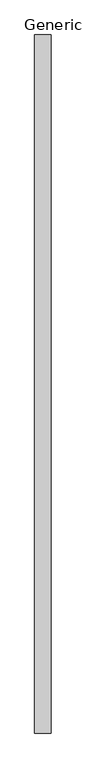
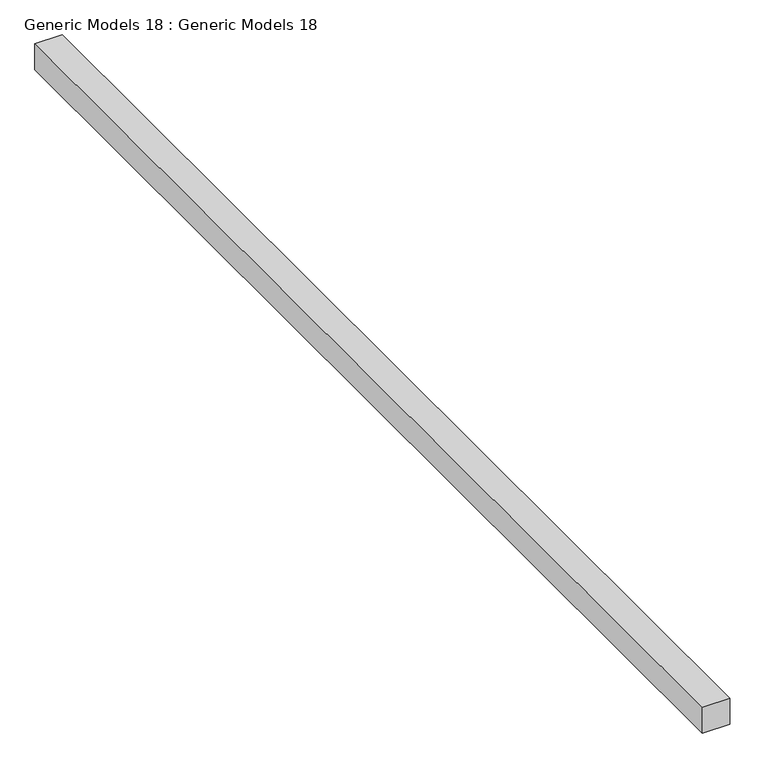
"""IFC4 building model written with IfcOpenShell, lengths in millimetres: proxy geometry, Generic Models 18 : Generic Models 18."""

from ifc_helpers import new_model, si_unit, frame, origin, place, context, project, spatial, polyline, outline, extrude, source, transform, mapped, element, save


def generic_models_18_generic_models_18_cf5f2b29(model_context):
    return source(origin(), model_context, "Body", "SweptSolid", [
        extrude(outline(polyline([(-15581.438074, -5903.3213044), (-15581.438074, 6941.8014639), (-15276.638074, 6941.8014639), (-15276.638074, -5903.3213044), (-15581.438074, -5903.3213044)])), frame((0.0, 0.0, 19507.2), z_axis=(0.0, 0.0, 1.0), x_axis=(1.0, 0.0, 0.0)), (0.0, 0.0, 1.0), 304.8),
    ])


if __name__ == "__main__":
    model = new_model("IFC4")
    model_context = context("Model", 3, world=origin())
    ifc_project = project(units=[si_unit("LENGTHUNIT", "METRE", prefix="MILLI")], contexts=[model_context])
    site = spatial("IfcSite", under=ifc_project)
    building = spatial("IfcBuilding", under=site)
    placement = place(None, origin())
    generic_models_18_generic_models_18_shape = generic_models_18_generic_models_18_cf5f2b29(model_context)
    element("IfcBuildingElementProxy", 1, Name="Generic Models 18 : Generic Models 18", ObjectType="Generic Models 18 : Generic Models 18", at=placement, inside=building, context=model_context, shape_type="MappedRepresentation", body=[
        mapped(generic_models_18_generic_models_18_shape, transform((0.0, 0.0, 0.0), x_axis=(1.0, 0.0, 0.0), y_axis=(0.0, 1.0, 0.0), z_axis=(0.0, 0.0, 1.0))),
    ])
    save(model, "model.ifc")
